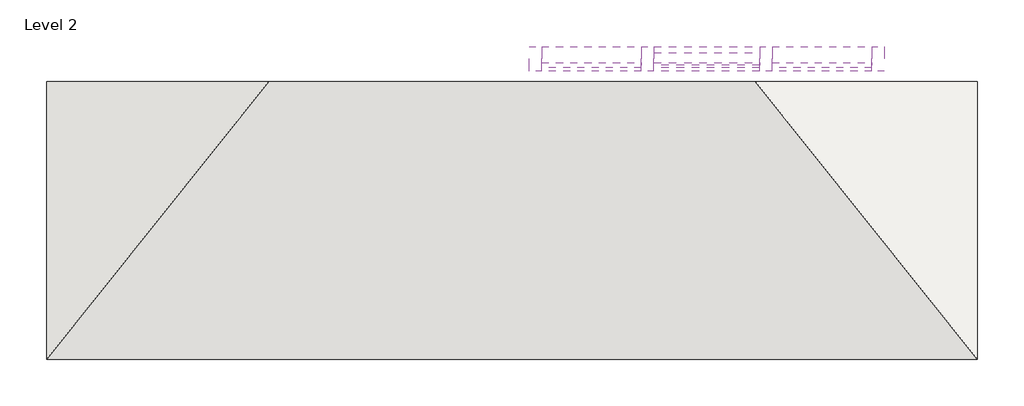
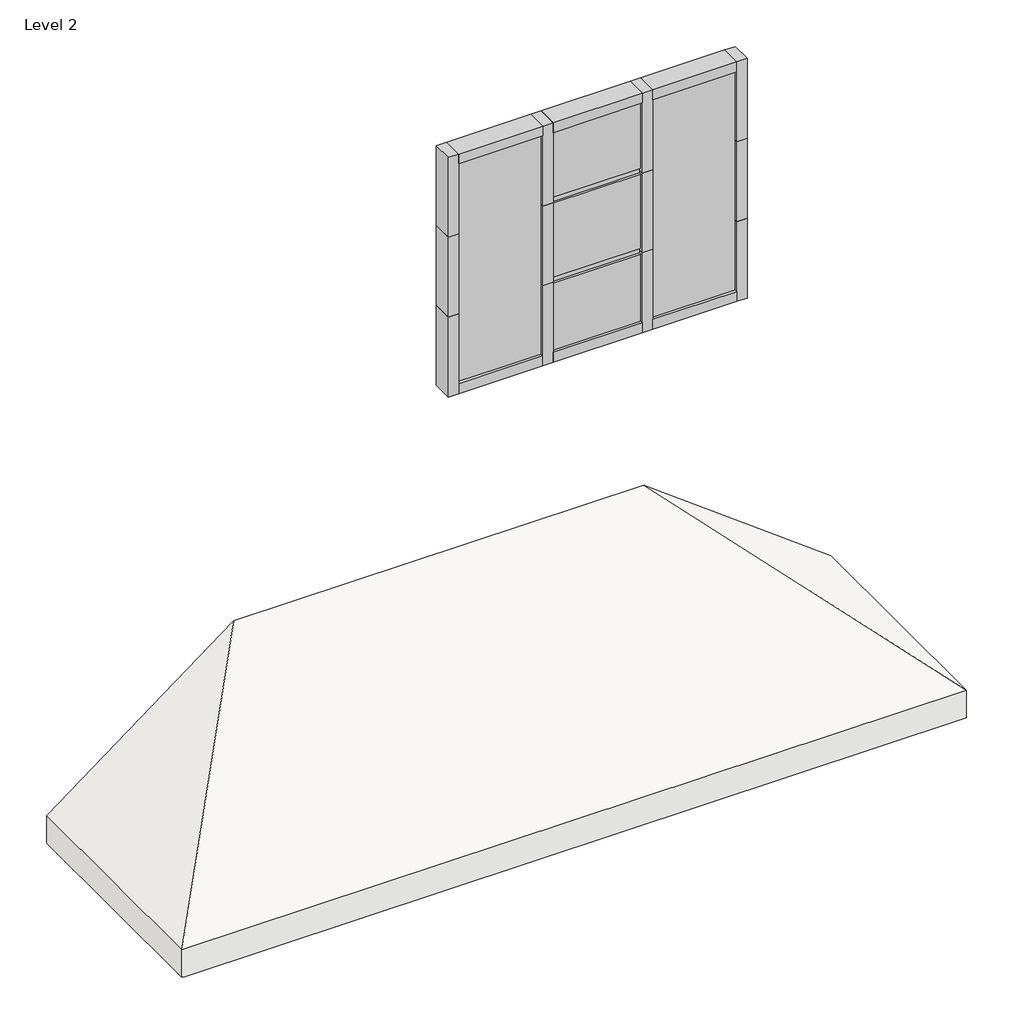
# One storey: 20 members, 5 plates, 1 roof.
"""IFC4 building model written with IfcOpenShell, lengths in millimetres."""

from ifc_helpers import new_model, si_unit, origin, place, context, project, spatial, faceted_brep, transform, mapped, element, save
from components import member_3578a4a6, member_0b7646a3, member_b3098cb3, member_a980948f, member_ce4f90f2, system_panel_glazed_f555cb13, system_panel_glazed_9e7866c3, system_panel_glazed_2ec405e4

model = new_model("IFC4")

# Units and contexts
model_context = context("Model", 3, world=origin())
ifc_project = project(units=[si_unit("LENGTHUNIT", "METRE", prefix="MILLI")], contexts=[model_context])

# Site, building, storey
site = spatial("IfcSite", under=ifc_project)
building = spatial("IfcBuilding", under=site)
storey = spatial("IfcBuildingStorey", under=building, Name="Level 2", Elevation=3657.6)

# Members
placement = place(None, origin())
member_shape = member_3578a4a6(model_context)
element("IfcMember", 1, ObjectType="Rectangular Mullion : 1.5\" x 2.5\" rectangular", at=placement, inside=storey, context=model_context, shape_type="MappedRepresentation", body=[
    mapped(member_shape, transform((-10560.0675664, -13837.7444793, 5909.7333333), x_axis=(0.0, 0.0, 1.0), y_axis=(0.0, 1.0, 0.0), z_axis=(-1.0, 0.0, 0.0))),
])
element("IfcMember", 2, ObjectType="Rectangular Mullion : 1.5\" x 2.5\" rectangular", at=placement, inside=storey, context=model_context, shape_type="MappedRepresentation", body=[
    mapped(member_shape, transform((-10560.0675664, -13837.7444793, 5393.2666667), x_axis=(0.0, 0.0, 1.0), y_axis=(0.0, 1.0, 0.0), z_axis=(-1.0, 0.0, 0.0))),
])
member_2_shape = member_0b7646a3(model_context)
element("IfcMember", 3, ObjectType="Rectangular Mullion : 2.5\" x 5\" rectangular", at=placement, inside=storey, context=model_context, shape_type="MappedRepresentation", body=[
    mapped(member_2_shape, transform((-11137.9175664, -13837.7444793, 6426.2), x_axis=(0.0, 0.0, 1.0), y_axis=(0.0, 1.0, 0.0), z_axis=(-1.0, 0.0, 0.0))),
])
element("IfcMember", 4, ObjectType="Rectangular Mullion : 2.5\" x 5\" rectangular", at=placement, inside=storey, context=model_context, shape_type="MappedRepresentation", body=[
    mapped(member_2_shape, transform((-9950.4675664, -13837.7444793, 6426.2), x_axis=(0.0, 0.0, 1.0), y_axis=(0.0, 1.0, 0.0), z_axis=(-1.0, 0.0, 0.0))),
])
element("IfcMember", 5, ObjectType="Rectangular Mullion : 2.5\" x 5\" rectangular", at=placement, inside=storey, context=model_context, shape_type="MappedRepresentation", body=[
    mapped(member_2_shape, transform((-9436.1175664, -13837.7444793, 4876.8), x_axis=(0.0, 0.0, -1.0), y_axis=(0.0, 1.0, 0.0), z_axis=(1.0, 0.0, 0.0))),
])
element("IfcMember", 6, ObjectType="Rectangular Mullion : 2.5\" x 5\" rectangular", at=placement, inside=storey, context=model_context, shape_type="MappedRepresentation", body=[
    mapped(member_2_shape, transform((-10623.5675664, -13837.7444793, 4876.8), x_axis=(0.0, 0.0, -1.0), y_axis=(0.0, 1.0, 0.0), z_axis=(1.0, 0.0, 0.0))),
])
member_3_shape = member_b3098cb3(model_context)
element("IfcMember", 7, ObjectType="Rectangular Mullion : 2.5\" x 5\" rectangular", at=placement, inside=storey, context=model_context, shape_type="MappedRepresentation", body=[
    mapped(member_3_shape, transform((-10591.8175664, -13837.7444793, 4876.8), x_axis=(-1.0, 0.0, 0.0), y_axis=(0.0, 1.0, 0.0), z_axis=(0.0, 0.0, -1.0))),
])
element("IfcMember", 8, ObjectType="Rectangular Mullion : 2.5\" x 5\" rectangular", at=placement, inside=storey, context=model_context, shape_type="MappedRepresentation", body=[
    mapped(member_3_shape, transform((-9982.2175664, -13837.7444793, 4876.8), x_axis=(-1.0, 0.0, 0.0), y_axis=(0.0, 1.0, 0.0), z_axis=(0.0, 0.0, -1.0))),
])
member_4_shape = member_a980948f(model_context)
element("IfcMember", 9, ObjectType="Rectangular Mullion : 2.5\" x 5\" rectangular", at=placement, inside=storey, context=model_context, shape_type="MappedRepresentation", body=[
    mapped(member_4_shape, transform((-10013.9675664, -13837.7444793, 4876.8), x_axis=(0.0, 0.0, -1.0), y_axis=(0.0, 1.0, 0.0), z_axis=(1.0, 0.0, 0.0))),
])
element("IfcMember", 10, ObjectType="Rectangular Mullion : 2.5\" x 5\" rectangular", at=placement, inside=storey, context=model_context, shape_type="MappedRepresentation", body=[
    mapped(member_4_shape, transform((-10560.0675664, -13837.7444793, 6426.2), x_axis=(0.0, 0.0, 1.0), y_axis=(0.0, 1.0, 0.0), z_axis=(-1.0, 0.0, 0.0))),
])
element("IfcMember", 11, ObjectType="Rectangular Mullion : 2.5\" x 5\" rectangular", at=placement, inside=storey, context=model_context, shape_type="MappedRepresentation", body=[
    mapped(member_3_shape, transform((-10591.8175664, -13837.7444793, 5909.7333333), x_axis=(-1.0, 0.0, 0.0), y_axis=(0.0, 1.0, 0.0), z_axis=(0.0, 0.0, -1.0))),
])
element("IfcMember", 12, ObjectType="Rectangular Mullion : 2.5\" x 5\" rectangular", at=placement, inside=storey, context=model_context, shape_type="MappedRepresentation", body=[
    mapped(member_3_shape, transform((-9982.2175664, -13837.7444793, 5909.7333333), x_axis=(-1.0, 0.0, 0.0), y_axis=(0.0, 1.0, 0.0), z_axis=(0.0, 0.0, -1.0))),
])
element("IfcMember", 13, ObjectType="Rectangular Mullion : 2.5\" x 5\" rectangular", at=placement, inside=storey, context=model_context, shape_type="MappedRepresentation", body=[
    mapped(member_3_shape, transform((-10591.8175664, -13837.7444793, 5393.2666667), x_axis=(-1.0, 0.0, 0.0), y_axis=(0.0, 1.0, 0.0), z_axis=(0.0, 0.0, -1.0))),
])
element("IfcMember", 14, ObjectType="Rectangular Mullion : 2.5\" x 5\" rectangular", at=placement, inside=storey, context=model_context, shape_type="MappedRepresentation", body=[
    mapped(member_3_shape, transform((-9982.2175664, -13837.7444793, 5393.2666667), x_axis=(-1.0, 0.0, 0.0), y_axis=(0.0, 1.0, 0.0), z_axis=(0.0, 0.0, -1.0))),
])
member_5_shape = member_ce4f90f2(model_context)
element("IfcMember", 15, ObjectType="Rectangular Mullion : 2.5\" x 5\" rectangular", at=placement, inside=storey, context=model_context, shape_type="MappedRepresentation", body=[
    mapped(member_5_shape, transform((-9372.6175664, -13837.7444793, 6426.2), x_axis=(1.0, 0.0, 0.0), y_axis=(0.0, 1.0, 0.0), z_axis=(0.0, 0.0, 1.0))),
])
element("IfcMember", 16, ObjectType="Rectangular Mullion : 2.5\" x 5\" rectangular", at=placement, inside=storey, context=model_context, shape_type="MappedRepresentation", body=[
    mapped(member_5_shape, transform((-11201.4175664, -13837.7444793, 4876.8), x_axis=(-1.0, 0.0, 0.0), y_axis=(0.0, 1.0, 0.0), z_axis=(0.0, 0.0, -1.0))),
])
element("IfcMember", 17, ObjectType="Rectangular Mullion : 2.5\" x 5\" rectangular", at=placement, inside=storey, context=model_context, shape_type="MappedRepresentation", body=[
    mapped(member_5_shape, transform((-11201.4175664, -13837.7444793, 5909.7333333), x_axis=(-1.0, 0.0, 0.0), y_axis=(0.0, 1.0, 0.0), z_axis=(0.0, 0.0, -1.0))),
])
element("IfcMember", 18, ObjectType="Rectangular Mullion : 2.5\" x 5\" rectangular", at=placement, inside=storey, context=model_context, shape_type="MappedRepresentation", body=[
    mapped(member_5_shape, transform((-11201.4175664, -13837.7444793, 5393.2666667), x_axis=(-1.0, 0.0, 0.0), y_axis=(0.0, 1.0, 0.0), z_axis=(0.0, 0.0, -1.0))),
])
element("IfcMember", 19, ObjectType="Rectangular Mullion : 2.5\" x 5\" rectangular", at=placement, inside=storey, context=model_context, shape_type="MappedRepresentation", body=[
    mapped(member_5_shape, transform((-9372.6175664, -13837.7444793, 5909.7333333), x_axis=(1.0, 0.0, 0.0), y_axis=(0.0, 1.0, 0.0), z_axis=(0.0, 0.0, 1.0))),
])
element("IfcMember", 20, ObjectType="Rectangular Mullion : 2.5\" x 5\" rectangular", at=placement, inside=storey, context=model_context, shape_type="MappedRepresentation", body=[
    mapped(member_5_shape, transform((-9372.6175664, -13837.7444793, 5393.2666667), x_axis=(1.0, 0.0, 0.0), y_axis=(0.0, 1.0, 0.0), z_axis=(0.0, 0.0, 1.0))),
])

# Plates
system_panel_glazed_shape = system_panel_glazed_f555cb13(model_context)
element("IfcPlate", 21, ObjectType="System Panel : Glazed", at=placement, inside=storey, context=model_context, shape_type="MappedRepresentation", body=[
    mapped(system_panel_glazed_shape, transform((-9693.2925664, -13837.7444793, 4940.3), x_axis=(-1.0, 0.0, 0.0), y_axis=(0.0, -1.0, 0.0), z_axis=(0.0, 0.0, 1.0))),
])
element("IfcPlate", 22, ObjectType="System Panel : Glazed", at=placement, inside=storey, context=model_context, shape_type="MappedRepresentation", body=[
    mapped(system_panel_glazed_shape, transform((-10880.7425664, -13837.7444793, 4940.3), x_axis=(-1.0, 0.0, 0.0), y_axis=(0.0, -1.0, 0.0), z_axis=(0.0, 0.0, 1.0))),
])
system_panel_glazed_2_shape = system_panel_glazed_9e7866c3(model_context)
element("IfcPlate", 23, ObjectType="System Panel : Glazed", at=placement, inside=storey, context=model_context, shape_type="MappedRepresentation", body=[
    mapped(system_panel_glazed_2_shape, transform((-10287.0175664, -13837.7444793, 4940.3), x_axis=(-1.0, 0.0, 0.0), y_axis=(0.0, -1.0, 0.0), z_axis=(0.0, 0.0, 1.0))),
])
element("IfcPlate", 24, ObjectType="System Panel : Glazed", at=placement, inside=storey, context=model_context, shape_type="MappedRepresentation", body=[
    mapped(system_panel_glazed_2_shape, transform((-10287.0175664, -13837.7444793, 5928.7833333), x_axis=(-1.0, 0.0, 0.0), y_axis=(0.0, -1.0, 0.0), z_axis=(0.0, 0.0, 1.0))),
])
system_panel_glazed_3_shape = system_panel_glazed_2ec405e4(model_context)
element("IfcPlate", 25, ObjectType="System Panel : Glazed", at=placement, inside=storey, context=model_context, shape_type="MappedRepresentation", body=[
    mapped(system_panel_glazed_3_shape, transform((-10287.0175664, -13837.7444793, 5412.3166667), x_axis=(-1.0, 0.0, 0.0), y_axis=(0.0, -1.0, 0.0), z_axis=(0.0, 0.0, 1.0))),
])

# Roof
element("IfcRoof", 26, ObjectType="roof 6\"", at=placement, inside=storey, context=model_context, shape_type="Brep", body=[
    faceted_brep([(-13673.3084236, -15388.1103416, 2895.6), (-12528.7748254, -13954.5978416, 3754.0001987), (-10053.1385958, -13954.5978416, 3754.0001987), (-8908.6049975, -15388.1103416, 2895.6), (-13673.3084236, -13954.5978416, 2895.6), (-8908.6049975, -13954.5978416, 2895.6), (-13690.4629606, -15388.1103416, 3073.2340973), (-8891.4504606, -15388.1103416, 3073.2340973), (-10035.9840589, -13954.5978416, 3931.634296), (-12545.9293623, -13954.5978416, 3931.634296), (-13690.4629606, -13954.5978416, 3073.2340973), (-8891.4504606, -13954.5978416, 3073.2340973), (-8891.4504606, -13954.5978416, 2895.6), (-8891.4504606, -15388.1103416, 2895.6), (-13690.4629606, -15388.1103416, 2895.6), (-13690.4629606, -13954.5978416, 2895.6)], [[[0, 1, 2, 3]], [[0, 4, 1]], [[2, 5, 3]], [[6, 7, 8, 9]], [[10, 6, 9]], [[11, 8, 7]], [[12, 11, 7, 13]], [[14, 6, 10, 15]], [[13, 7, 6, 14, 0, 3]], [[12, 13, 3, 5]], [[10, 9, 8, 11, 12, 5, 2, 1, 4, 15]], [[0, 14, 15, 4]]]),
])

save(model, "model.ifc")

# Revit data of these elements
# Type "Rectangular Mullion : 1.5\" x 2.5\" rectangular"
#   built-in parameter 1007304 = 0.208333 (stored number, unit not read)
#   built-in parameter 1007301 = 0.0625 (stored number, unit not read)
#   built-in parameter 1007300 = 0.0625 (stored number, unit not read)
# Type "Rectangular Mullion : 2.5\" x 5\" rectangular"
#   built-in parameter 1007304 = 0.416667 (stored number, unit not read)
#   built-in parameter 1007301 = 0.104167 (stored number, unit not read)
#   built-in parameter 1007300 = 0.104167 (stored number, unit not read)
# Type "System Panel : Glazed"
#   Construction Type Id = "GSP4R"
#   Analytic Construction = "1/8 in Pilkington single glazing"
#   Visual Light Transmittance = 0.9
#   Solar Heat Gain Coefficient = 0.86
#   Heat Transfer Coefficient (U) = 1.18115 BTU/(h·ft²·°F)
#   Define Thermal Properties by = 1
# Type "roof 6\""
#   Assembly Code = "B1020"
#   Layers, outside or top first: 0' - 6" "ROOF" (function 1)
# Elements 1, 2 (IfcMember, "Rectangular Mullion : 1.5\" x 2.5\" rectangular")
#   Phase Created = New Construction
#   Materials on its faces: "Aluminum"
# Elements 3, 4, 5, 6, 7, 8, 9, 10, 11, 12, 13, 14, 15, 16, 17, 18, 19, 20 (IfcMember, "Rectangular Mullion : 2.5\" x 5\" rectangular")
#   Phase Created = New Construction
# Elements 21, 22, 23, 24, 25 (IfcPlate, "System Panel : Glazed")
#   Phase Created = New Construction
#   Materials on its faces: "Glass"
# Element 26 (IfcRoof, "roof 6\"")
#   built-in parameter 1001705 = 12.8991 (stored number, unit not read)
#   built-in parameter 1001701 = -2.5 (stored number, unit not read)
#   built-in parameter 1001710 = 33615
#   Phase Created = New Construction
#   Materials on its faces: "ROOF"
# Materials
#   "ROOF": class "Generic", colour RGB 120 120 120, transparency 0, Cost = 0
#   "Aluminum": class "Metal", colour RGB 247 247 247, transparency 0, Description = "Aluminum 6061", Cost = 0
#   "Glass": class "Glass", colour RGB 0 128 192, transparency 0.75, Description = "Soda Lime Glass", Cost = 0
